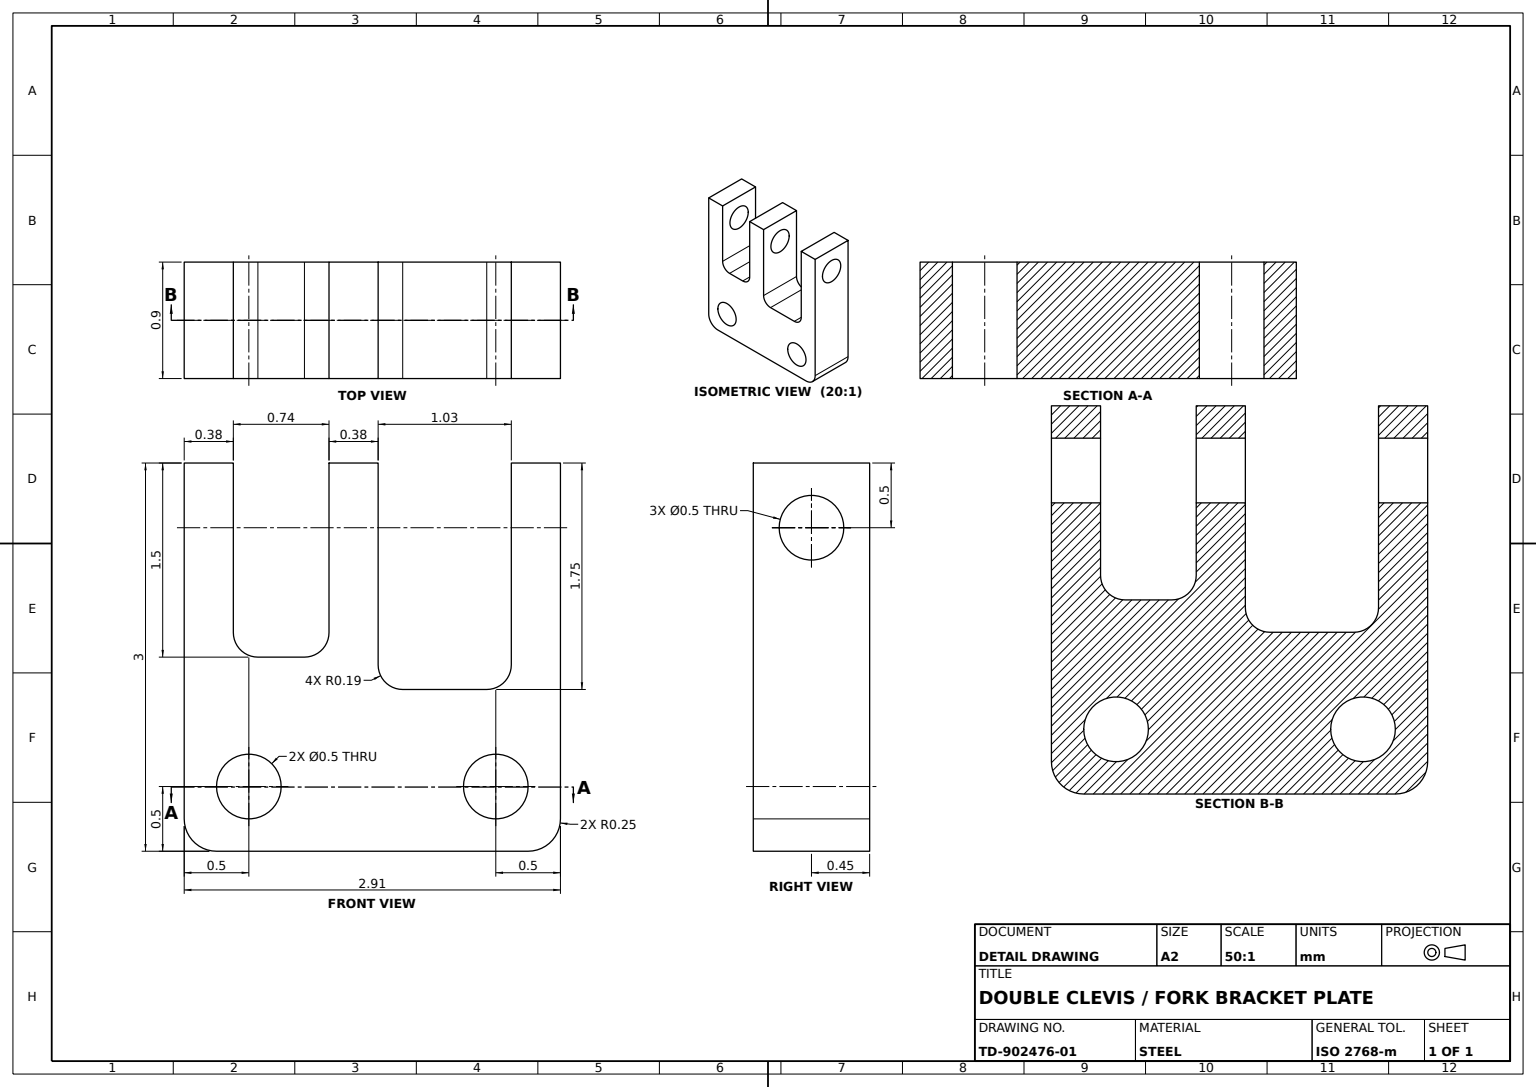
SolidWorks part; units mm, degrees
material "Plain Carbon Steel"
ref_plane "Front Plane" through (0, 0, 0) normal (0, 0, 1) x (1, 0, 0)
ref_plane "Top Plane" through (0, 0, 0) normal (0, 1, 0) x (1, 0, 0)
ref_plane "Right Plane" through (0, 0, 0) normal (1, 0, 0) x (0, 0, -1)
sketch "Bracket Plate Profile" plane through (0, 0, 0) normal (0, 1, 0) x (1, 0, 0)
  line L1 (-1.455, -0.45) -> (1.455, -0.45)
  line L2 (-1.455, -0.45) -> (-1.455, 0.45)
  line L3 (-1.455, 0.45) -> (1.455, 0.45)
  line L4 (1.455, -0.45) -> (1.455, 0.45)
  line L5 (-1.455, -0.45) -> (1.455, 0.45) construction
  line L6 (-1.455, 0.45) -> (1.455, -0.45) construction
  point P0 (0, 0)
  dimension "D1" = 0.9
  dimension "D2" = 2.91
extrude "Bracket Plate" add sketch "Bracket Plate Profile" along normal blind 3
fillet "Corner Fillet R0.25" radius 0.25 2 edges at (1.455, 0, 0) (-1.455, 0, 0)
sketch "Prong Slots Sketch" plane through (0, 0, 0.45) normal (0, 0, 1) x (1, 0, 0)
  line L0 (-1.075, 3) -> (-1.075, 1.69)
  line L1 (-1.455, 3) -> (1.455, 3) construction
  line L2 (1.075, 3) -> (1.075, 1.44)
  line L3 (0.885, 1.25) -> (0.235, 1.25)
  line L4 (0.045, 1.44) -> (0.045, 3)
  line L5 (1.455, 3) -> (1.455, 0.25) construction
  line L6 (-1.455, 3) -> (-1.455, 0.25) construction
  line L7 (-0.885, 1.5) -> (-0.525, 1.5)
  line L8 (-0.335, 1.69) -> (-0.335, 3)
  line L9 (-1.075, 3) -> (-0.335, 3)
  line L10 (0.045, 3) -> (1.075, 3)
  arc A0 (1.075, 1.44) -> (0.885, 1.25) centre (0.885, 1.44) cw
  arc A1 (0.235, 1.25) -> (0.045, 1.44) centre (0.235, 1.44) cw
  arc A2 (-0.525, 1.5) -> (-0.335, 1.69) centre (-0.525, 1.69) ccw
  arc A3 (-1.075, 1.69) -> (-0.885, 1.5) centre (-0.885, 1.69) ccw
  point P16 (1.075, 1.25)
  point P19 (0.045, 1.25)
  point P24 (-1.075, 1.5)
  dimension "D7" = 0.19
  dimension "D1" = 0.38
  dimension "D2" = 1.03
  dimension "D3" = 1.75
  dimension "D4" = 0.38
  dimension "D5" = 0.38
  dimension "D6" = 1.5
extrude "Prong Slots" cut sketch "Prong Slots Sketch" against normal blind 3
sketch "Mounting Holes Sketch" plane through (0, 0, 0.45) normal (0, 0, 1) x (1, 0, 0)
  line L0 (-1.205, 0) -> (1.205, 0) construction
  line L1 (-1.455, 3) -> (-1.455, 0.25) construction
  line L2 (1.455, 3) -> (1.455, 0.25) construction
  circle A0 centre (-0.955, 0.5) radius 0.25
  circle A1 centre (0.955, 0.5) radius 0.25
  dimension "D1" = 0.5
  dimension "D2" = 0.5
  dimension "D3" = 0.5
  dimension "D4" = 0.5
  dimension "D5" = 0.5
  dimension "D6" = 0.5
extrude "Mounting Holes 2x" cut sketch "Mounting Holes Sketch" against normal blind 3
sketch "Cross Pin Bore Sketch" plane through (1.455, 0, 0) normal (1, 0, 0) x (0, 0, -1)
  line L0 (-0.45, 3) -> (-0.45, 0.25) construction
  line L1 (-0.45, 3) -> (0.45, 3) construction
  circle A0 centre (0, 2.5) radius 0.25
  dimension "D1" = 0.5
  dimension "D2" = 0.45
  dimension "D3" = 0.5
extrude "Cross Pin Bore" cut sketch "Cross Pin Bore Sketch" against normal through all
